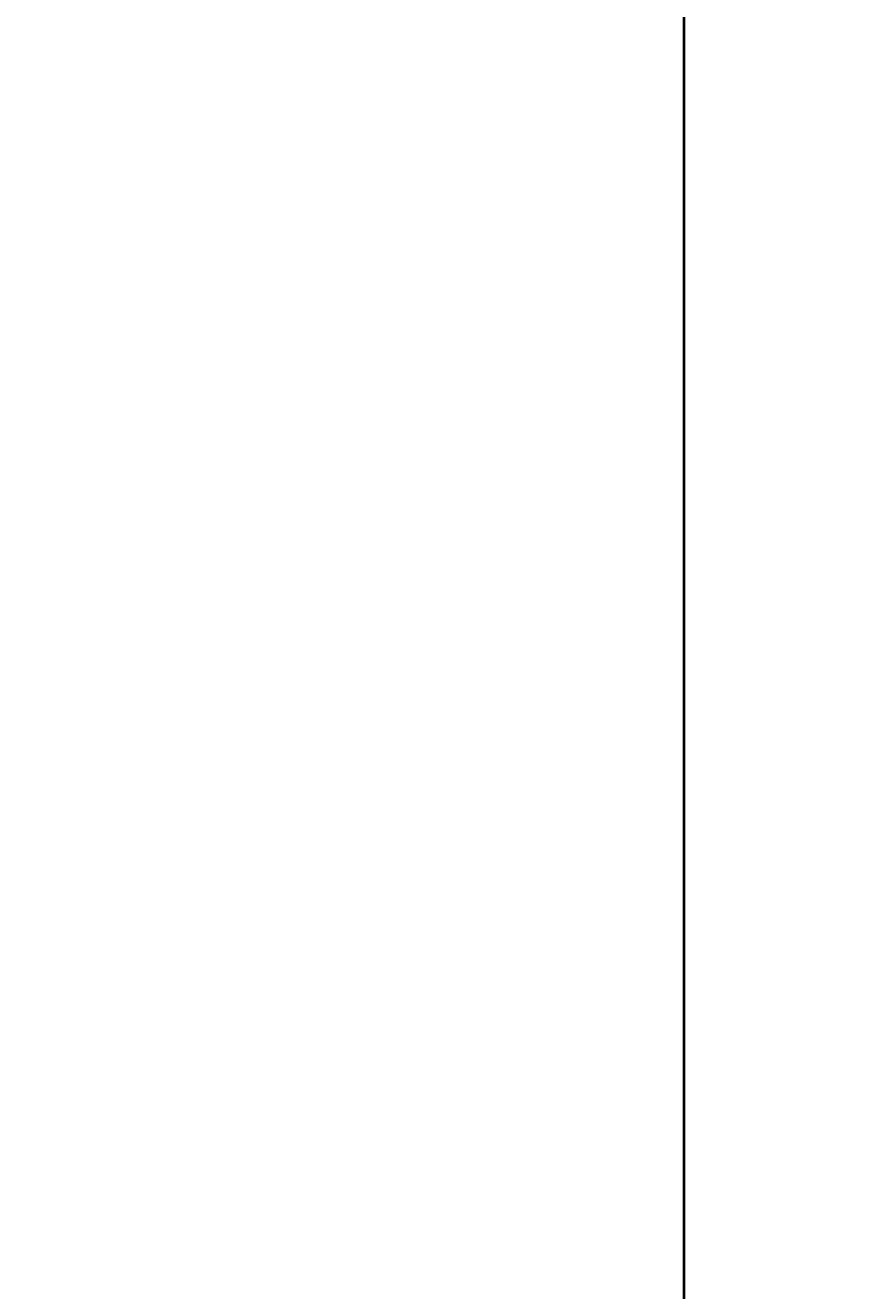
# Model space of a CAD drawing. Units: millimetres. Extents: x 27017497 to 27018854, y 7058029 to 7059154.
# Tile 57 of 91: x 27018010 to 27018038, y 7058327 to 7058369. Entities that reach past the tile are written whole.
import ezdxf

# ---------------------------------------------------------------- set-up
doc = ezdxf.new("R2010")
doc.units = ezdxf.units.MM
doc.layers.add('A-ANNO-DIMS', color=2, linetype='Continuous', lineweight=18)
doc.layers.add('A-WALL', color=7, linetype='Continuous', lineweight=35)
doc.styles.get("Standard").update_dxf_attribs({"font": 'arial.ttf'})
doc.dimstyles.get("Standard").update_dxf_attribs({"dimtxt": 0.18, "dimasz": 0.18, "dimexe": 0.18, "dimexo": 0.0625, "dimgap": 0.09, "dimtad": 0, "dimtih": 1, "dimtoh": 1, "dimdec": 4, "dimzin": 0, "dimdsep": 46, "dimtxsty": 'Standard', "dimcen": 0.09, "dimadec": 0, "dimazin": 0, "dimtfac": 1, "dimtdec": 4, "dimtofl": 0, "dimtmove": 0, "dimatfit": 3, "dimfxl": 1, "dimtolj": 1, "dimtzin": 0, "dimarcsym": 0})

# ---------------------------------------------------------------- blocks, each defined once
blk = doc.blocks.new('*D48')
at = {"layer": 'A-ANNO-DIMS', "color": 0, "lineweight": -2, "transparency": 16777216}
for p, q in [((27018463.498, 7058622.912), (27017497.536, 7058622.912)), ((27017497.716, 7058622.732), (27017497.716, 7058357.753)), ((27017497.716, 7058092.41), (27017497.716, 7058357.389)), ((27018555.129, 7058092.23), (27017497.536, 7058092.23))]:
    blk.add_line(p, q, dxfattribs=at)
at = {"layer": 'A-ANNO-DIMS', "color": 0, "transparency": 16777216}
for points in [[(27017497.686, 7058622.732), (27017497.746, 7058622.732), (27017497.716, 7058622.912)], [(27017497.686, 7058092.41), (27017497.746, 7058092.41), (27017497.716, 7058092.23)]]:
    blk.add_solid(points, dxfattribs=at)
at = {"layer": 'Defpoints', "color": 0, "transparency": 16777216}
for p in [(27018463.561, 7058622.912), (27017497.716, 7058092.23), (27018555.192, 7058092.23)]:
    blk.add_point(p, dxfattribs=at)
at = {"layer": 'A-ANNO-DIMS', "color": 0, "transparency": 16777216, "insert": (27017497.716, 7058357.571), "char_height": 0.18, "attachment_point": 5}
blk.add_mtext('\\A1;530.7', dxfattribs=at)

msp = doc.modelspace()

# ---------------------------------------------------------------- linework, layer by layer
at = {"layer": 'A-WALL'}
msp.add_line((27018032.166, 7058386.803), (27018032.166, 7058141.912), dxfattribs=at)
msp.add_lwpolyline([(27018032.178, 7058237.363), (27018032.178, 7058375.363)], dxfattribs=at)

# ---------------------------------------------------------------- dimensions: what is measured, and where the dimension line sits
at = {"layer": 'A-ANNO-DIMS'}
dim = msp.add_linear_dim(base=(27017497.716, 7058092.23), p1=(27018463.561, 7058622.912), p2=(27018555.192, 7058092.23), angle=90, dimstyle='Standard', override={"dimdec": 1, "dimlfac": 1, "dimrnd": 0, "dimzin": 0, "dimdsep": 46, "dimlunit": 2}, dxfattribs=at)
dim.commit()
dim.dimension.update_dxf_attribs({"geometry": '*D48', "text_midpoint": (27017497.716, 7058357.571)})

doc.saveas('drawing.dxf')
